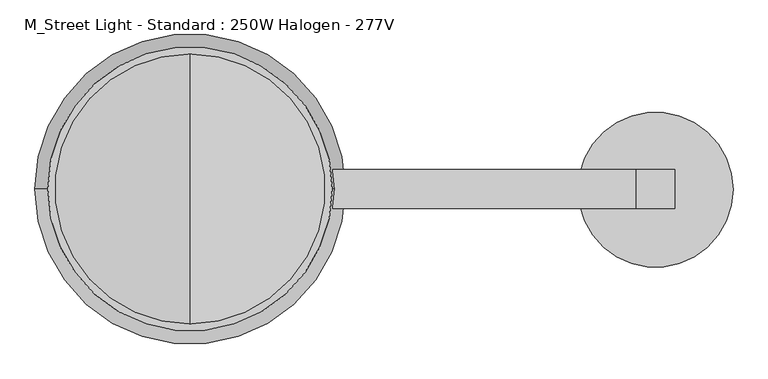
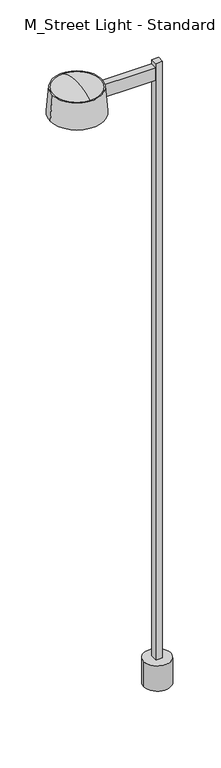
"""IFC4 building model written with IfcOpenShell, lengths in millimetres: light fixture geometry, M_Street Light - Standard : 250W Halogen - 277V."""

from ifc_helpers import new_model, si_unit, point, frame, origin, origin_with_axes, origin_2d, place, context, project, spatial, polyline, circle_curve, ellipse_curve, trimmed, segment, composite_curve, outline, extrude, source, transform, mapped, element, save
from ifc_brep_helpers import plane_surface, revolved_surface, advanced_brep


def m_street_light_standard_250w_halogen_277v_204dbcbb(model_context):
    return source(origin(), model_context, "Body", "SolidModel", [
        extrude(outline(composite_curve([segment(trimmed(circle_curve(origin_2d(), 152.4), [point((-152.4, 0.0))], [point((152.4, 0.0))], False, "CARTESIAN"), True, "CONTINUOUS"), segment(trimmed(circle_curve(origin_2d(), 152.4), [point((152.4, 0.0))], [point((-152.4, 0.0))], False, "CARTESIAN"), True, "CONTINUOUS")], self_intersect=False)), origin_with_axes(), (0.0, 0.0, 1.0), 304.8),
        extrude(outline(polyline([(38.1, 38.1), (38.1, -38.1), (-38.1, -38.1), (-38.1, 38.1), (38.1, 38.1)])), frame((0.0, 0.0, 304.8), z_axis=(0.0, 0.0, 1.0), x_axis=(1.0, 0.0, 0.0)), (0.0, 0.0, 1.0), 7195.2),
        extrude(outline(polyline([(-914.4, 38.1), (-38.1, 38.1), (-38.1, -38.1), (-914.4, -38.1), (-914.4, 38.1)])), frame((0.0, 0.0, 7296.8), z_axis=(0.0, 0.0, 1.0), x_axis=(1.0, 0.0, 0.0)), (0.0, 0.0, 1.0), 152.4),
        advanced_brep(
        [(-1193.8, 0.0, 7500.0), (-635.0, 0.0, 7500.0), (-1219.2, 0.0, 7195.2), (-609.6, 0.0, 7195.2)],
        [
            (0, 1, circle_curve(frame((-914.4, 0.0, 7500.0), z_axis=(0.0, 0.0, 1.0), x_axis=(-1.0, 0.0, 0.0)), 279.4)),
            (1, 0, circle_curve(frame((-914.4, 0.0, 7500.0), z_axis=(0.0, 0.0, 1.0), x_axis=(1.0, 0.0, 0.0)), 279.4)),
            (2, 3, circle_curve(frame((-914.4, 0.0, 7195.2), z_axis=(0.0, 0.0, -1.0), x_axis=(1.0, 0.0, 0.0)), 304.8)),
            (3, 2, circle_curve(frame((-914.4, 0.0, 7195.2), z_axis=(0.0, 0.0, -1.0), x_axis=(-1.0, 0.0, 0.0)), 304.8)),
            (3, 1),
            (0, 2),
        ],
        [
            plane_surface(frame((-914.4, 0.0, 7500.0), z_axis=(0.0, 0.0, 1.0), x_axis=(0.0, -1.0, 0.0))),
            plane_surface(frame((-914.4, 0.0, 7195.2), z_axis=(0.0, 0.0, -1.0), x_axis=(0.0, -1.0, 0.0))),
            revolved_surface(polyline([(-1193.8, 0.0, 7500.0), (-1219.2, 0.0, 7195.2)]), (-914.4, 0.0, 10852.8), (0.0, 0.0, -1.0)),
            revolved_surface(polyline([(-635.0, 0.0, 7500.0), (-609.6, 0.0, 7195.2)]), (-914.4, 0.0, 10852.8), (0.0, 0.0, -1.0)),
        ],
        [
            (0, [[1, 2]]),
            (1, [[3, 4]]),
            (2, [[-4, 5, -1, 6]]),
            (3, [[-3, -6, -2, -5]]),
        ],
    ),
        advanced_brep(
        [(-914.4, -266.7, 7500.0), (-914.4, 266.7, 7500.0), (-914.4, 0.0, 7571.4620496), (-914.4, -228.6332063, 7500.0), (-914.4, 228.6332063, 7500.0), (-914.4, 0.0, 7558.7620496)],
        [
            (0, 1, circle_curve(frame((-914.4, 0.0, 7500.0), z_axis=(0.0, 0.0, 1.0), x_axis=(0.0, 1.0, 0.0)), 266.7)),
            (1, 2, circle_curve(frame((-914.4, -28.9924067, 6929.8609147), z_axis=(1.0, 0.0, 0.0), x_axis=(0.0, 0.0, 1.0)), 642.2558493)),
            (2, 0, circle_curve(frame((-914.4, 28.9924067, 6929.8609147), z_axis=(1.0, 0.0, 0.0), x_axis=(0.0, 0.0, 1.0)), 642.2558493)),
            (1, 0, circle_curve(frame((-914.4, 0.0, 7500.0), z_axis=(0.0, 0.0, 1.0), x_axis=(0.0, 1.0, 0.0)), 266.7)),
            (3, 4, circle_curve(frame((-914.4, 0.0, 7500.0), z_axis=(0.0, 0.0, 1.0), x_axis=(0.0, 1.0, 0.0)), 228.6332063)),
            (4, 1),
            (0, 3),
            (4, 3, circle_curve(frame((-914.4, 0.0, 7500.0), z_axis=(0.0, 0.0, 1.0), x_axis=(0.0, 1.0, 0.0)), 228.6332063)),
            (5, 4),
            (3, 5),
        ],
        [
            revolved_surface(trimmed(ellipse_curve(frame((-914.4, -28.9924067, 6929.8609147), z_axis=(-1.0, 0.0, 0.0), x_axis=(0.0, 0.0, 1.0)), 642.2558493, 642.2558493), [point((-914.4, 0.0, 7571.4620496))], [point((-914.4, 266.7, 7500.0))], True, "CARTESIAN"), (-914.4, 0.0, 7423.8), (0.0, 0.0, -1.0)),
            plane_surface(frame((-914.4, 0.0, 7500.0), z_axis=(0.0, 0.0, -1.0), x_axis=(0.0, 1.0, 0.0))),
            revolved_surface(polyline([(-914.4, 228.6332063, 7500.0), (-914.4, 0.0, 7558.7620496)]), (-914.4, 0.0, 7423.8), (0.0, 0.0, -1.0)),
        ],
        [
            (0, [[1, 2, 3]]),
            (0, [[4, -3, -2]]),
            (1, [[5, 6, -1, 7]]),
            (1, [[8, -7, -4, -6]]),
            (2, [[9, -5, 10]]),
            (2, [[-10, -8, -9]]),
        ],
    ),
        advanced_brep(
        [(-914.4, -228.6332063, 7195.2), (-914.4, 228.6332063, 7195.2), (-914.4, 0.0, 7136.4379504), (-914.4, -266.7, 7195.2), (-914.4, 266.7, 7195.2), (-914.4, 0.0, 7123.7379504)],
        [
            (0, 1, circle_curve(frame((-914.4, 0.0, 7195.2), z_axis=(0.0, 0.0, 1.0), x_axis=(0.0, 1.0, 0.0)), 228.6332063)),
            (1, 2),
            (2, 0),
            (1, 0, circle_curve(frame((-914.4, 0.0, 7195.2), z_axis=(0.0, 0.0, 1.0), x_axis=(0.0, 1.0, 0.0)), 228.6332063)),
            (3, 4, circle_curve(frame((-914.4, 0.0, 7195.2), z_axis=(0.0, 0.0, 1.0), x_axis=(0.0, 1.0, 0.0)), 266.7)),
            (4, 1),
            (0, 3),
            (4, 3, circle_curve(frame((-914.4, 0.0, 7195.2), z_axis=(0.0, 0.0, 1.0), x_axis=(0.0, 1.0, 0.0)), 266.7)),
            (5, 4, circle_curve(frame((-914.4, -28.9924067, 7765.3390853), z_axis=(1.0, 0.0, 0.0), x_axis=(0.0, 0.0, -1.0)), 642.2558493)),
            (3, 5, circle_curve(frame((-914.4, 28.9924067, 7765.3390853), z_axis=(1.0, 0.0, 0.0), x_axis=(0.0, 0.0, -1.0)), 642.2558493)),
        ],
        [
            revolved_surface(polyline([(-914.4, 0.0, 7136.4379504), (-914.4, 228.6332063, 7195.2)]), (-914.4, 0.0, 7271.4), (0.0, 0.0, -1.0)),
            plane_surface(frame((-914.4, 0.0, 7195.2), z_axis=(0.0, 0.0, 1.0), x_axis=(0.0, 1.0, 0.0))),
            revolved_surface(trimmed(ellipse_curve(frame((-914.4, -28.9924067, 7765.3390853), z_axis=(-1.0, 0.0, 0.0), x_axis=(0.0, 0.0, -1.0)), 642.2558493, 642.2558493), [point((-914.4, 266.7, 7195.2))], [point((-914.4, 0.0, 7123.7379504))], True, "CARTESIAN"), (-914.4, 0.0, 7271.4), (0.0, 0.0, -1.0)),
        ],
        [
            (0, [[1, 2, 3]]),
            (0, [[4, -3, -2]]),
            (1, [[5, 6, -1, 7]]),
            (1, [[8, -7, -4, -6]]),
            (2, [[9, -5, 10]]),
            (2, [[-10, -8, -9]]),
        ],
    ),
    ])


if __name__ == "__main__":
    model = new_model("IFC4")
    model_context = context("Model", 3, world=origin())
    ifc_project = project(units=[si_unit("LENGTHUNIT", "METRE", prefix="MILLI")], contexts=[model_context])
    site = spatial("IfcSite", under=ifc_project)
    building = spatial("IfcBuilding", under=site)
    placement = place(None, origin())
    m_street_light_standard_250w_halogen_277v_shape = m_street_light_standard_250w_halogen_277v_204dbcbb(model_context)
    element("IfcLightFixture", 1, ObjectType="M_Street Light - Standard : 250W Halogen - 277V", at=placement, inside=building, context=model_context, shape_type="MappedRepresentation", body=[
        mapped(m_street_light_standard_250w_halogen_277v_shape, transform((0.0, 0.0, 0.0), x_axis=(1.0, 0.0, 0.0), y_axis=(0.0, 1.0, 0.0), z_axis=(0.0, 0.0, 1.0))),
    ])
    save(model, "model.ifc")

# Revit data of these elements
# Type "M_Street Light - Standard : 250W Halogen - 277V"
#   Photometric Web File = "SLS1T4.IES"
#   Lamp = "T-4"
#   Wattage Comments = "250"
#   Wattage = 250 W
#   built-in parameter 1150110 = 1 (stored number, unit not read)
#   built-in parameter 1114217 = 1 (stored number, unit not read)
#   built-in parameter 1150109 = 1 (stored number, unit not read)
#   built-in parameter 1150113 = 1 (stored number, unit not read)
#   Tilt Angle = -90.00°
#   built-in parameter 1150115 = 1 (stored number, unit not read)
#   built-in parameter 1150105 = 397.887 (stored number, unit not read)
#   built-in parameter 1150112 = 1 (stored number, unit not read)
#   built-in parameter 1150114 = 1 (stored number, unit not read)
#   built-in parameter 1150107 = 3200 (stored number, unit not read)
#   built-in parameter 1150106 = 3.97887 (stored number, unit not read)
#   Height = 7500 mm
#   Lumens = 5000 lm
#   built-in parameter 1150104 = 1.85806 (stored number, unit not read)
#   Voltage = 277 V
#   built-in parameter 1114218 = 1 (stored number, unit not read)
#   built-in parameter 1150133 = 10 (stored number, unit not read)
#   Apparent Load = 250 VA
#   built-in parameter 1150134 = 3
#   built-in parameter 1150137 = 1
#   Color Filter = 16777215
#   Number of poles = 1
#   Stand Material = Steel, Paint Finish, Dark Gray, Matte
#   Shade Material = Steel, Paint Finish, Dark Gray, Matte
#   Load Classification = Lighting - Exterior
#   Diffuser Material = Glass, Frosted
#   Dimming Lamp Color Temperature Shift = (empty or 0)
#   Default Elevation = 0
# Element 1 (IfcLightFixture, "M_Street Light - Standard : 250W Halogen - 277V")
#   Materials on its faces: "Steel, Paint Finish, Dark Gray, Matte", "Glass, Frosted"
# Materials
#   "Steel, Paint Finish, Dark Gray, Matte": class "Metal", colour RGB 0 0 0, transparency 0, Description = "Steel, paint finish, dark gray, matte", Cost = 0
#   "Glass, Frosted": class "Glass", colour RGB 249 250 249, transparency 0.8, Description = "physical material", Cost = 0
